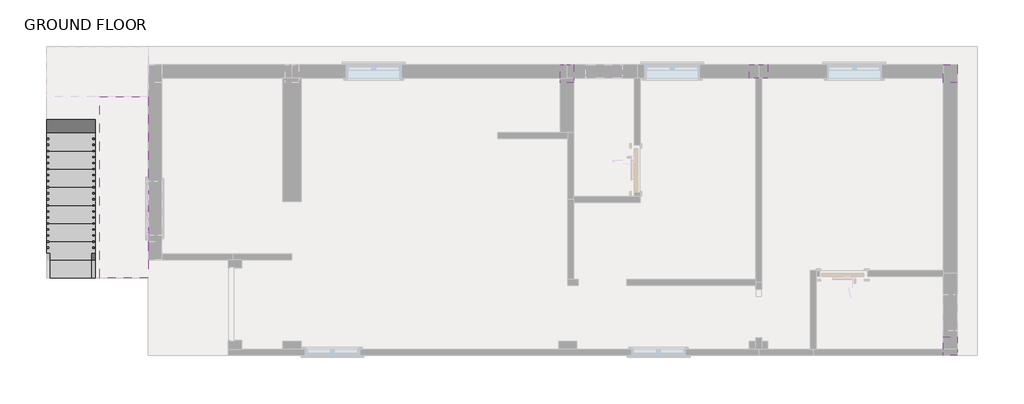
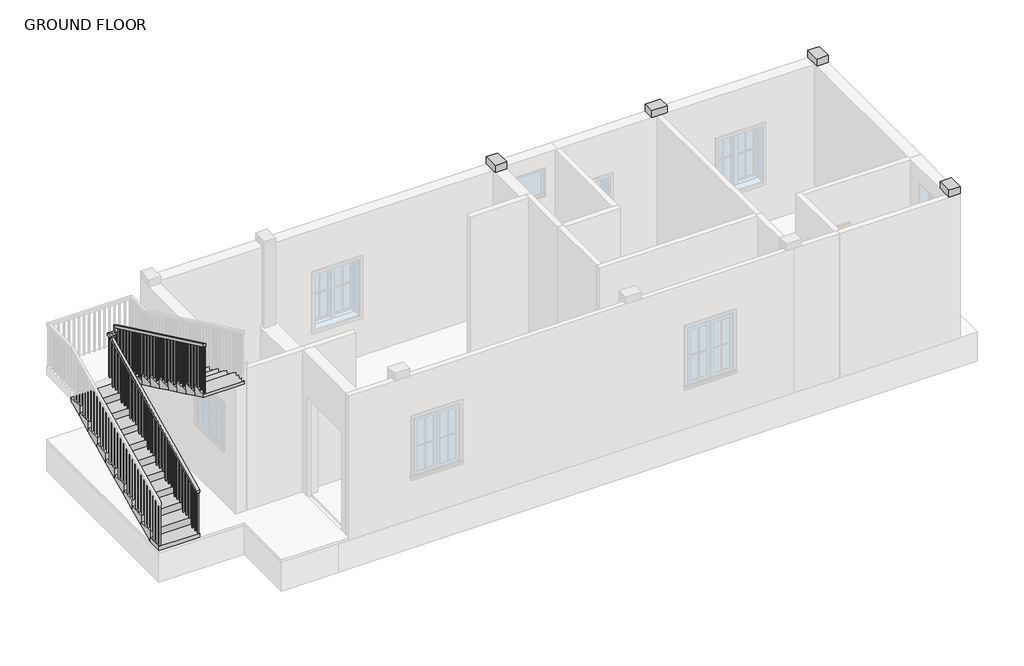
# One storey, part 2 of 3: 4 columns, 2 stair flights, 1 railing.
"""IFC4 building model written with IfcOpenShell, lengths in millimetres."""

from ifc_helpers import new_model, si_unit, frame, origin, place, context, project, spatial, polyline, outline, extrude, faceted_brep, element, save

model = new_model("IFC4")

# Units and contexts
model_context = context("Model", 3, world=origin())
ifc_project = project(units=[si_unit("LENGTHUNIT", "METRE", prefix="MILLI")], contexts=[model_context])

# Site, building, storey
site = spatial("IfcSite", under=ifc_project)
building = spatial("IfcBuilding", under=site)
storey = spatial("IfcBuildingStorey", under=building, Name="GROUND FLOOR", Elevation=0.0)

# Columns
placement = place(None, origin())
element("IfcColumn", 1, ObjectType="Rectangular Column : 9\" X 12\"", at=placement, inside=storey, context=model_context, shape_type="SweptSolid", body=[
    extrude(outline(polyline([(8641.6408773, 5102.5642852), (8870.2408773, 5102.5642852), (8870.2408773, 4797.7642852), (8641.6408773, 4797.7642852), (8641.6408773, 5102.5642852)])), frame((0.0, 0.0, 3048.0), z_axis=(0.0, 0.0, 1.0), x_axis=(1.0, 0.0, 0.0)), (0.0, 0.0, 1.0), 152.4),
])
element("IfcColumn", 2, ObjectType="Rectangular Column : 9\" X 12\"", at=placement, inside=storey, context=model_context, shape_type="SweptSolid", body=[
    extrude(outline(polyline([(3200.4, 5695.2408773), (3200.4, 5390.4408773), (3048.0, 5390.4408773), (3048.0, 5542.8408773), (3048.0, 5695.2408773), (3200.4, 5695.2408773)])), frame((0.0, 4873.9642852, 0.0), z_axis=(0.0, 1.0, 0.0), x_axis=(0.0, 0.0, 1.0)), (0.0, 0.0, 1.0), 228.6),
])
element("IfcColumn", 3, ObjectType="Rectangular Column : 9\" X 12\"", at=placement, inside=storey, context=model_context, shape_type="Brep", body=[
    faceted_brep([(2215.4408773, 5102.5642852, 3200.4), (2444.0408773, 5102.5642852, 3200.4), (2444.0408773, 5102.5642852, 3048.0), (2329.7408773, 5102.5642852, 3048.0), (2215.4408773, 5102.5642852, 3048.0), (2444.0408773, 4797.7642852, 3200.4), (2444.0408773, 4797.7642852, 3048.0), (2444.0408773, 4873.9642852, 3048.0), (2215.4408773, 4797.7642852, 3200.4), (2215.4408773, 4797.7642852, 3048.0), (2215.4408773, 4873.9642852, 3048.0), (2329.7408773, 4873.9642852, 3048.0)], [[[0, 1, 2, 3, 4]], [[1, 5, 6, 7, 2]], [[5, 8, 9, 6]], [[8, 0, 4, 10, 9]], [[1, 0, 8, 5]], [[6, 9, 10, 11, 7]], [[10, 4, 3, 11]], [[3, 2, 7, 11]]]),
])
element("IfcColumn", 4, ObjectType="Rectangular Column : 9\" X 12\"", at=placement, inside=storey, context=model_context, shape_type="SweptSolid", body=[
    extrude(outline(polyline([(225.7642852, 3200.4), (530.5642852, 3200.4), (530.5642852, 3048.0), (327.3642852, 3048.0), (225.7642852, 3048.0), (225.7642852, 3200.4)])), frame((8641.6408773, 0.0, 0.0), z_axis=(1.0, 0.0, 0.0), x_axis=(0.0, 1.0, 0.0)), (0.0, 0.0, 1.0), 228.6),
])

# Railing
element("IfcRailing", 5, ObjectType="Handrail - Rectangular", at=placement, inside=storey, context=model_context, shape_type="SolidModel", body=[
    faceted_brep([(-5633.1591227, 1521.1642852, 1059.8727273), (-5633.1591227, 1521.1642852, 1003.5834559), (-5582.3591227, 1521.1642852, 1003.5834559), (-5582.3591227, 1521.1642852, 1059.8727273), (-5633.1591227, 4492.9642852, 2478.2318182), (-5633.1591227, 4543.7642852, 2446.1880014), (-5582.3591227, 4543.7642852, 2446.1880014), (-5582.3591227, 4492.9642852, 2478.2318182), (-5633.1591227, 4492.9642852, 2514.6), (-5633.1591227, 4543.7642852, 2463.8), (-5582.3591227, 4543.7642852, 2463.8), (-5582.3591227, 4492.9642852, 2514.6), (-5633.1591227, 4619.9642852, 2514.6), (-5633.1591227, 4619.9642852, 2463.8), (-5582.3591227, 4569.1642852, 2463.8), (-5582.3591227, 4569.1642852, 2514.6), (-5506.1591227, 4619.9642852, 2514.6), (-5506.1591227, 4619.9642852, 2463.8), (-5506.1591227, 4569.1642852, 2463.8), (-5506.1591227, 4569.1642852, 2514.6), (-5480.7591227, 4619.9642852, 2514.6), (-5480.7591227, 4569.1642852, 2514.6), (-5480.7591227, 4569.1642852, 2463.8), (-5480.7591227, 4619.9642852, 2463.8)], [[[0, 1, 2, 3]], [[1, 0, 4, 5]], [[2, 1, 5, 6]], [[3, 2, 6, 7]], [[0, 3, 7, 4]], [[5, 4, 8, 9]], [[6, 5, 9, 10]], [[7, 6, 10, 11]], [[4, 7, 11, 8]], [[9, 8, 12, 13]], [[10, 9, 13, 14]], [[11, 10, 14, 15]], [[8, 11, 15, 12]], [[13, 12, 16, 17]], [[14, 13, 17, 18]], [[15, 14, 18, 19]], [[12, 15, 19, 16]], [[20, 21, 22, 23]], [[17, 16, 20, 23]], [[18, 17, 23, 22]], [[19, 18, 22, 21]], [[16, 19, 21, 20]]]),
    faceted_brep([(-5506.1591227, 4619.9642852, 2514.6), (-5455.3591227, 4619.9642852, 2463.8), (-5455.3591227, 4569.1642852, 2463.8), (-5506.1591227, 4569.1642852, 2514.6), (-5506.1591227, 4619.9642852, 2635.8272727), (-5506.1591227, 4569.1642852, 2603.7834559), (-5455.3591227, 4569.1642852, 2603.7834559), (-5455.3591227, 4619.9642852, 2635.8272727)], [[[0, 1, 2, 3]], [[4, 5, 6, 7]], [[1, 0, 4, 7]], [[2, 1, 7, 6]], [[3, 2, 6, 5]], [[0, 3, 5, 4]]]),
    faceted_brep([(-5455.3591227, 4619.9642852, 2635.8272727), (-5455.3591227, 4569.1642852, 2603.7834559), (-5506.1591227, 4569.1642852, 2603.7834559), (-5506.1591227, 4619.9642852, 2635.8272727), (-5455.3591227, 1521.1642852, 4114.8), (-5506.1591227, 1521.1642852, 4114.8), (-5506.1591227, 1521.1642852, 4058.5107287), (-5455.3591227, 1521.1642852, 4058.5107287)], [[[0, 1, 2, 3]], [[4, 5, 6, 7]], [[1, 0, 4, 7]], [[2, 1, 7, 6]], [[3, 2, 6, 5]], [[0, 3, 5, 4]]]),
    extrude(outline(polyline([(1537.0392852, 4050.9340241), (1556.0892852, 4041.8419787), (1556.0892852, 3054.9272727), (1537.0392852, 3054.9272727), (1537.0392852, 4050.9340241)])), frame((-5490.2841227, 0.0, 0.0), z_axis=(1.0, 0.0, 0.0), x_axis=(0.0, 1.0, 0.0)), (0.0, 0.0, 1.0), 19.05),
    extrude(outline(polyline([(1638.6392852, 4002.443115), (1657.6892852, 3993.3510696), (1657.6892852, 3054.9272727), (1638.6392852, 3054.9272727), (1638.6392852, 4002.443115)])), frame((-5490.2841227, 0.0, 0.0), z_axis=(1.0, 0.0, 0.0), x_axis=(0.0, 1.0, 0.0)), (0.0, 0.0, 1.0), 19.05),
    extrude(outline(polyline([(1740.2392852, 3953.9522059), (1759.2892852, 3944.8601605), (1759.2892852, 3054.9272727), (1740.2392852, 3054.9272727), (1740.2392852, 3953.9522059)])), frame((-5490.2841227, 0.0, 0.0), z_axis=(1.0, 0.0, 0.0), x_axis=(0.0, 1.0, 0.0)), (0.0, 0.0, 1.0), 19.05),
    extrude(outline(polyline([(1841.8392852, 3905.4612969), (1860.8892852, 3896.3692514), (1860.8892852, 2909.4545455), (1841.8392852, 2909.4545455), (1841.8392852, 3905.4612969)])), frame((-5490.2841227, 0.0, 0.0), z_axis=(1.0, 0.0, 0.0), x_axis=(0.0, 1.0, 0.0)), (0.0, 0.0, 1.0), 19.05),
    extrude(outline(polyline([(1943.4392852, 3856.9703878), (1962.4892852, 3847.8783423), (1962.4892852, 2909.4545455), (1943.4392852, 2909.4545455), (1943.4392852, 3856.9703878)])), frame((-5490.2841227, 0.0, 0.0), z_axis=(1.0, 0.0, 0.0), x_axis=(0.0, 1.0, 0.0)), (0.0, 0.0, 1.0), 19.05),
    extrude(outline(polyline([(2045.0392852, 3808.4794787), (2064.0892852, 3799.3874332), (2064.0892852, 2909.4545455), (2045.0392852, 2909.4545455), (2045.0392852, 3808.4794787)])), frame((-5490.2841227, 0.0, 0.0), z_axis=(1.0, 0.0, 0.0), x_axis=(0.0, 1.0, 0.0)), (0.0, 0.0, 1.0), 19.05),
    extrude(outline(polyline([(2146.6392852, 3759.9885696), (2165.6892852, 3750.8965241), (2165.6892852, 2763.9818182), (2146.6392852, 2763.9818182), (2146.6392852, 3759.9885696)])), frame((-5490.2841227, 0.0, 0.0), z_axis=(1.0, 0.0, 0.0), x_axis=(0.0, 1.0, 0.0)), (0.0, 0.0, 1.0), 19.05),
    extrude(outline(polyline([(2248.2392852, 3711.4976605), (2267.2892852, 3702.405615), (2267.2892852, 2763.9818182), (2248.2392852, 2763.9818182), (2248.2392852, 3711.4976605)])), frame((-5490.2841227, 0.0, 0.0), z_axis=(1.0, 0.0, 0.0), x_axis=(0.0, 1.0, 0.0)), (0.0, 0.0, 1.0), 19.05),
    extrude(outline(polyline([(2349.8392852, 3663.0067514), (2368.8892852, 3653.9147059), (2368.8892852, 2763.9818182), (2349.8392852, 2763.9818182), (2349.8392852, 3663.0067514)])), frame((-5490.2841227, 0.0, 0.0), z_axis=(1.0, 0.0, 0.0), x_axis=(0.0, 1.0, 0.0)), (0.0, 0.0, 1.0), 19.05),
    extrude(outline(polyline([(2451.4392852, 3614.5158423), (2470.4892852, 3605.4237969), (2470.4892852, 2618.5090909), (2451.4392852, 2618.5090909), (2451.4392852, 3614.5158423)])), frame((-5490.2841227, 0.0, 0.0), z_axis=(1.0, 0.0, 0.0), x_axis=(0.0, 1.0, 0.0)), (0.0, 0.0, 1.0), 19.05),
    extrude(outline(polyline([(2553.0392852, 3566.0249332), (2572.0892852, 3556.9328878), (2572.0892852, 2618.5090909), (2553.0392852, 2618.5090909), (2553.0392852, 3566.0249332)])), frame((-5490.2841227, 0.0, 0.0), z_axis=(1.0, 0.0, 0.0), x_axis=(0.0, 1.0, 0.0)), (0.0, 0.0, 1.0), 19.05),
    extrude(outline(polyline([(2654.6392852, 3517.5340241), (2673.6892852, 3508.4419787), (2673.6892852, 2618.5090909), (2654.6392852, 2618.5090909), (2654.6392852, 3517.5340241)])), frame((-5490.2841227, 0.0, 0.0), z_axis=(1.0, 0.0, 0.0), x_axis=(0.0, 1.0, 0.0)), (0.0, 0.0, 1.0), 19.05),
    extrude(outline(polyline([(2756.2392852, 3469.043115), (2775.2892852, 3459.9510696), (2775.2892852, 2473.0363636), (2756.2392852, 2473.0363636), (2756.2392852, 3469.043115)])), frame((-5490.2841227, 0.0, 0.0), z_axis=(1.0, 0.0, 0.0), x_axis=(0.0, 1.0, 0.0)), (0.0, 0.0, 1.0), 19.05),
    extrude(outline(polyline([(2857.8392852, 3420.5522059), (2876.8892852, 3411.4601605), (2876.8892852, 2473.0363636), (2857.8392852, 2473.0363636), (2857.8392852, 3420.5522059)])), frame((-5490.2841227, 0.0, 0.0), z_axis=(1.0, 0.0, 0.0), x_axis=(0.0, 1.0, 0.0)), (0.0, 0.0, 1.0), 19.05),
    extrude(outline(polyline([(2959.4392852, 3372.0612969), (2978.4892852, 3362.9692514), (2978.4892852, 2473.0363636), (2959.4392852, 2473.0363636), (2959.4392852, 3372.0612969)])), frame((-5490.2841227, 0.0, 0.0), z_axis=(1.0, 0.0, 0.0), x_axis=(0.0, 1.0, 0.0)), (0.0, 0.0, 1.0), 19.05),
    extrude(outline(polyline([(3061.0392852, 3323.5703878), (3080.0892852, 3314.4783423), (3080.0892852, 2327.5636364), (3061.0392852, 2327.5636364), (3061.0392852, 3323.5703878)])), frame((-5490.2841227, 0.0, 0.0), z_axis=(1.0, 0.0, 0.0), x_axis=(0.0, 1.0, 0.0)), (0.0, 0.0, 1.0), 19.05),
    extrude(outline(polyline([(3162.6392852, 3275.0794787), (3181.6892852, 3265.9874332), (3181.6892852, 2327.5636364), (3162.6392852, 2327.5636364), (3162.6392852, 3275.0794787)])), frame((-5490.2841227, 0.0, 0.0), z_axis=(1.0, 0.0, 0.0), x_axis=(0.0, 1.0, 0.0)), (0.0, 0.0, 1.0), 19.05),
    extrude(outline(polyline([(3264.2392852, 3226.5885696), (3283.2892852, 3217.4965241), (3283.2892852, 2327.5636364), (3264.2392852, 2327.5636364), (3264.2392852, 3226.5885696)])), frame((-5490.2841227, 0.0, 0.0), z_axis=(1.0, 0.0, 0.0), x_axis=(0.0, 1.0, 0.0)), (0.0, 0.0, 1.0), 19.05),
    extrude(outline(polyline([(3365.8392852, 3178.0976605), (3384.8892852, 3169.005615), (3384.8892852, 2182.0909091), (3365.8392852, 2182.0909091), (3365.8392852, 3178.0976605)])), frame((-5490.2841227, 0.0, 0.0), z_axis=(1.0, 0.0, 0.0), x_axis=(0.0, 1.0, 0.0)), (0.0, 0.0, 1.0), 19.05),
    extrude(outline(polyline([(3467.4392852, 3129.6067514), (3486.4892852, 3120.5147059), (3486.4892852, 2182.0909091), (3467.4392852, 2182.0909091), (3467.4392852, 3129.6067514)])), frame((-5490.2841227, 0.0, 0.0), z_axis=(1.0, 0.0, 0.0), x_axis=(0.0, 1.0, 0.0)), (0.0, 0.0, 1.0), 19.05),
    extrude(outline(polyline([(3569.0392852, 3081.1158423), (3588.0892852, 3072.0237969), (3588.0892852, 2182.0909091), (3569.0392852, 2182.0909091), (3569.0392852, 3081.1158423)])), frame((-5490.2841227, 0.0, 0.0), z_axis=(1.0, 0.0, 0.0), x_axis=(0.0, 1.0, 0.0)), (0.0, 0.0, 1.0), 19.05),
    extrude(outline(polyline([(3670.6392852, 3032.6249332), (3689.6892852, 3023.5328878), (3689.6892852, 2036.6181818), (3670.6392852, 2036.6181818), (3670.6392852, 3032.6249332)])), frame((-5490.2841227, 0.0, 0.0), z_axis=(1.0, 0.0, 0.0), x_axis=(0.0, 1.0, 0.0)), (0.0, 0.0, 1.0), 19.05),
    extrude(outline(polyline([(3772.2392852, 2984.1340241), (3791.2892852, 2975.0419787), (3791.2892852, 2036.6181818), (3772.2392852, 2036.6181818), (3772.2392852, 2984.1340241)])), frame((-5490.2841227, 0.0, 0.0), z_axis=(1.0, 0.0, 0.0), x_axis=(0.0, 1.0, 0.0)), (0.0, 0.0, 1.0), 19.05),
    extrude(outline(polyline([(3873.8392852, 2935.643115), (3892.8892852, 2926.5510696), (3892.8892852, 2036.6181818), (3873.8392852, 2036.6181818), (3873.8392852, 2935.643115)])), frame((-5490.2841227, 0.0, 0.0), z_axis=(1.0, 0.0, 0.0), x_axis=(0.0, 1.0, 0.0)), (0.0, 0.0, 1.0), 19.05),
    extrude(outline(polyline([(3975.4392852, 2887.1522059), (3994.4892852, 2878.0601605), (3994.4892852, 1891.1454545), (3975.4392852, 1891.1454545), (3975.4392852, 2887.1522059)])), frame((-5490.2841227, 0.0, 0.0), z_axis=(1.0, 0.0, 0.0), x_axis=(0.0, 1.0, 0.0)), (0.0, 0.0, 1.0), 19.05),
    extrude(outline(polyline([(4077.0392852, 2838.6612969), (4096.0892852, 2829.5692514), (4096.0892852, 1891.1454545), (4077.0392852, 1891.1454545), (4077.0392852, 2838.6612969)])), frame((-5490.2841227, 0.0, 0.0), z_axis=(1.0, 0.0, 0.0), x_axis=(0.0, 1.0, 0.0)), (0.0, 0.0, 1.0), 19.05),
    extrude(outline(polyline([(4178.6392852, 2790.1703878), (4197.6892852, 2781.0783423), (4197.6892852, 1891.1454545), (4178.6392852, 1891.1454545), (4178.6392852, 2790.1703878)])), frame((-5490.2841227, 0.0, 0.0), z_axis=(1.0, 0.0, 0.0), x_axis=(0.0, 1.0, 0.0)), (0.0, 0.0, 1.0), 19.05),
    extrude(outline(polyline([(4280.2392852, 2741.6794787), (4299.2892852, 2732.5874332), (4299.2892852, 1745.6727273), (4280.2392852, 1745.6727273), (4280.2392852, 2741.6794787)])), frame((-5490.2841227, 0.0, 0.0), z_axis=(1.0, 0.0, 0.0), x_axis=(0.0, 1.0, 0.0)), (0.0, 0.0, 1.0), 19.05),
    extrude(outline(polyline([(4381.8392852, 2693.1885696), (4400.8892852, 2684.0965241), (4400.8892852, 1745.6727273), (4381.8392852, 1745.6727273), (4381.8392852, 2693.1885696)])), frame((-5490.2841227, 0.0, 0.0), z_axis=(1.0, 0.0, 0.0), x_axis=(0.0, 1.0, 0.0)), (0.0, 0.0, 1.0), 19.05),
    extrude(outline(polyline([(4483.4392852, 2644.6976605), (4502.4892852, 2635.605615), (4502.4892852, 1745.6727273), (4483.4392852, 1745.6727273), (4483.4392852, 2644.6976605)])), frame((-5490.2841227, 0.0, 0.0), z_axis=(1.0, 0.0, 0.0), x_axis=(0.0, 1.0, 0.0)), (0.0, 0.0, 1.0), 19.05),
    extrude(outline(polyline([(-5515.6841227, 4585.0392852), (-5515.6841227, 4604.0892852), (-5496.6341227, 4604.0892852), (-5496.6341227, 4585.0392852), (-5515.6841227, 4585.0392852)])), frame((0.0, 0.0, 1600.2), z_axis=(0.0, 0.0, 1.0), x_axis=(1.0, 0.0, 0.0)), (0.0, 0.0, 1.0), 863.6),
    extrude(outline(polyline([(-5598.2341227, 4559.6392852), (-5617.2841227, 4559.6392852), (-5617.2841227, 4578.6892852), (-5598.2341227, 4578.6892852), (-5598.2341227, 4559.6392852)])), frame((0.0, 0.0, 1600.2), z_axis=(0.0, 0.0, 1.0), x_axis=(1.0, 0.0, 0.0)), (0.0, 0.0, 1.0), 863.6),
    extrude(outline(polyline([(4458.0392852, 2405.2737969), (4477.0892852, 2414.3658423), (4477.0892852, 1454.7272727), (4458.0392852, 1454.7272727), (4458.0392852, 2405.2737969)])), frame((-5617.2841227, 0.0, 0.0), z_axis=(1.0, 0.0, 0.0), x_axis=(0.0, 1.0, 0.0)), (0.0, 0.0, 1.0), 19.05),
    extrude(outline(polyline([(4356.4392852, 2356.7828878), (4375.4892852, 2365.8749332), (4375.4892852, 1454.7272727), (4356.4392852, 1454.7272727), (4356.4392852, 2356.7828878)])), frame((-5617.2841227, 0.0, 0.0), z_axis=(1.0, 0.0, 0.0), x_axis=(0.0, 1.0, 0.0)), (0.0, 0.0, 1.0), 19.05),
    extrude(outline(polyline([(4254.8392852, 2308.2919787), (4273.8892852, 2317.3840241), (4273.8892852, 1454.7272727), (4254.8392852, 1454.7272727), (4254.8392852, 2308.2919787)])), frame((-5617.2841227, 0.0, 0.0), z_axis=(1.0, 0.0, 0.0), x_axis=(0.0, 1.0, 0.0)), (0.0, 0.0, 1.0), 19.05),
    extrude(outline(polyline([(4153.2392852, 2259.8010696), (4172.2892852, 2268.893115), (4172.2892852, 1309.2545455), (4153.2392852, 1309.2545455), (4153.2392852, 2259.8010696)])), frame((-5617.2841227, 0.0, 0.0), z_axis=(1.0, 0.0, 0.0), x_axis=(0.0, 1.0, 0.0)), (0.0, 0.0, 1.0), 19.05),
    extrude(outline(polyline([(4051.6392852, 2211.3101605), (4070.6892852, 2220.4022059), (4070.6892852, 1309.2545455), (4051.6392852, 1309.2545455), (4051.6392852, 2211.3101605)])), frame((-5617.2841227, 0.0, 0.0), z_axis=(1.0, 0.0, 0.0), x_axis=(0.0, 1.0, 0.0)), (0.0, 0.0, 1.0), 19.05),
    extrude(outline(polyline([(3950.0392852, 2162.8192514), (3969.0892852, 2171.9112969), (3969.0892852, 1309.2545455), (3950.0392852, 1309.2545455), (3950.0392852, 2162.8192514)])), frame((-5617.2841227, 0.0, 0.0), z_axis=(1.0, 0.0, 0.0), x_axis=(0.0, 1.0, 0.0)), (0.0, 0.0, 1.0), 19.05),
    extrude(outline(polyline([(3848.4392852, 2114.3283423), (3867.4892852, 2123.4203878), (3867.4892852, 1163.7818182), (3848.4392852, 1163.7818182), (3848.4392852, 2114.3283423)])), frame((-5617.2841227, 0.0, 0.0), z_axis=(1.0, 0.0, 0.0), x_axis=(0.0, 1.0, 0.0)), (0.0, 0.0, 1.0), 19.05),
    extrude(outline(polyline([(3746.8392852, 2065.8374332), (3765.8892852, 2074.9294787), (3765.8892852, 1163.7818182), (3746.8392852, 1163.7818182), (3746.8392852, 2065.8374332)])), frame((-5617.2841227, 0.0, 0.0), z_axis=(1.0, 0.0, 0.0), x_axis=(0.0, 1.0, 0.0)), (0.0, 0.0, 1.0), 19.05),
    extrude(outline(polyline([(3645.2392852, 2017.3465241), (3664.2892852, 2026.4385696), (3664.2892852, 1163.7818182), (3645.2392852, 1163.7818182), (3645.2392852, 2017.3465241)])), frame((-5617.2841227, 0.0, 0.0), z_axis=(1.0, 0.0, 0.0), x_axis=(0.0, 1.0, 0.0)), (0.0, 0.0, 1.0), 19.05),
    extrude(outline(polyline([(3543.6392852, 1968.855615), (3562.6892852, 1977.9476605), (3562.6892852, 1018.3090909), (3543.6392852, 1018.3090909), (3543.6392852, 1968.855615)])), frame((-5617.2841227, 0.0, 0.0), z_axis=(1.0, 0.0, 0.0), x_axis=(0.0, 1.0, 0.0)), (0.0, 0.0, 1.0), 19.05),
    extrude(outline(polyline([(3442.0392852, 1920.3647059), (3461.0892852, 1929.4567514), (3461.0892852, 1018.3090909), (3442.0392852, 1018.3090909), (3442.0392852, 1920.3647059)])), frame((-5617.2841227, 0.0, 0.0), z_axis=(1.0, 0.0, 0.0), x_axis=(0.0, 1.0, 0.0)), (0.0, 0.0, 1.0), 19.05),
    extrude(outline(polyline([(3340.4392852, 1871.8737969), (3359.4892852, 1880.9658423), (3359.4892852, 1018.3090909), (3340.4392852, 1018.3090909), (3340.4392852, 1871.8737969)])), frame((-5617.2841227, 0.0, 0.0), z_axis=(1.0, 0.0, 0.0), x_axis=(0.0, 1.0, 0.0)), (0.0, 0.0, 1.0), 19.05),
    extrude(outline(polyline([(3238.8392852, 1823.3828878), (3257.8892852, 1832.4749332), (3257.8892852, 872.8363636), (3238.8392852, 872.8363636), (3238.8392852, 1823.3828878)])), frame((-5617.2841227, 0.0, 0.0), z_axis=(1.0, 0.0, 0.0), x_axis=(0.0, 1.0, 0.0)), (0.0, 0.0, 1.0), 19.05),
    extrude(outline(polyline([(3137.2392852, 1774.8919787), (3156.2892852, 1783.9840241), (3156.2892852, 872.8363636), (3137.2392852, 872.8363636), (3137.2392852, 1774.8919787)])), frame((-5617.2841227, 0.0, 0.0), z_axis=(1.0, 0.0, 0.0), x_axis=(0.0, 1.0, 0.0)), (0.0, 0.0, 1.0), 19.05),
    extrude(outline(polyline([(3035.6392852, 1726.4010696), (3054.6892852, 1735.493115), (3054.6892852, 872.8363636), (3035.6392852, 872.8363636), (3035.6392852, 1726.4010696)])), frame((-5617.2841227, 0.0, 0.0), z_axis=(1.0, 0.0, 0.0), x_axis=(0.0, 1.0, 0.0)), (0.0, 0.0, 1.0), 19.05),
    extrude(outline(polyline([(2934.0392852, 1677.9101605), (2953.0892852, 1687.0022059), (2953.0892852, 727.3636364), (2934.0392852, 727.3636364), (2934.0392852, 1677.9101605)])), frame((-5617.2841227, 0.0, 0.0), z_axis=(1.0, 0.0, 0.0), x_axis=(0.0, 1.0, 0.0)), (0.0, 0.0, 1.0), 19.05),
    extrude(outline(polyline([(2832.4392852, 1629.4192514), (2851.4892852, 1638.5112969), (2851.4892852, 727.3636364), (2832.4392852, 727.3636364), (2832.4392852, 1629.4192514)])), frame((-5617.2841227, 0.0, 0.0), z_axis=(1.0, 0.0, 0.0), x_axis=(0.0, 1.0, 0.0)), (0.0, 0.0, 1.0), 19.05),
    extrude(outline(polyline([(2730.8392852, 1580.9283423), (2749.8892852, 1590.0203878), (2749.8892852, 727.3636364), (2730.8392852, 727.3636364), (2730.8392852, 1580.9283423)])), frame((-5617.2841227, 0.0, 0.0), z_axis=(1.0, 0.0, 0.0), x_axis=(0.0, 1.0, 0.0)), (0.0, 0.0, 1.0), 19.05),
    extrude(outline(polyline([(2629.2392852, 1532.4374332), (2648.2892852, 1541.5294787), (2648.2892852, 581.8909091), (2629.2392852, 581.8909091), (2629.2392852, 1532.4374332)])), frame((-5617.2841227, 0.0, 0.0), z_axis=(1.0, 0.0, 0.0), x_axis=(0.0, 1.0, 0.0)), (0.0, 0.0, 1.0), 19.05),
    extrude(outline(polyline([(2527.6392852, 1483.9465241), (2546.6892852, 1493.0385696), (2546.6892852, 581.8909091), (2527.6392852, 581.8909091), (2527.6392852, 1483.9465241)])), frame((-5617.2841227, 0.0, 0.0), z_axis=(1.0, 0.0, 0.0), x_axis=(0.0, 1.0, 0.0)), (0.0, 0.0, 1.0), 19.05),
    extrude(outline(polyline([(2426.0392852, 1435.455615), (2445.0892852, 1444.5476605), (2445.0892852, 581.8909091), (2426.0392852, 581.8909091), (2426.0392852, 1435.455615)])), frame((-5617.2841227, 0.0, 0.0), z_axis=(1.0, 0.0, 0.0), x_axis=(0.0, 1.0, 0.0)), (0.0, 0.0, 1.0), 19.05),
    extrude(outline(polyline([(2324.4392852, 1386.9647059), (2343.4892852, 1396.0567514), (2343.4892852, 436.4181818), (2324.4392852, 436.4181818), (2324.4392852, 1386.9647059)])), frame((-5617.2841227, 0.0, 0.0), z_axis=(1.0, 0.0, 0.0), x_axis=(0.0, 1.0, 0.0)), (0.0, 0.0, 1.0), 19.05),
    extrude(outline(polyline([(2222.8392852, 1338.4737969), (2241.8892852, 1347.5658423), (2241.8892852, 436.4181818), (2222.8392852, 436.4181818), (2222.8392852, 1338.4737969)])), frame((-5617.2841227, 0.0, 0.0), z_axis=(1.0, 0.0, 0.0), x_axis=(0.0, 1.0, 0.0)), (0.0, 0.0, 1.0), 19.05),
    extrude(outline(polyline([(2121.2392852, 1289.9828878), (2140.2892852, 1299.0749332), (2140.2892852, 436.4181818), (2121.2392852, 436.4181818), (2121.2392852, 1289.9828878)])), frame((-5617.2841227, 0.0, 0.0), z_axis=(1.0, 0.0, 0.0), x_axis=(0.0, 1.0, 0.0)), (0.0, 0.0, 1.0), 19.05),
    extrude(outline(polyline([(2019.6392852, 1241.4919787), (2038.6892852, 1250.5840241), (2038.6892852, 290.9454545), (2019.6392852, 290.9454545), (2019.6392852, 1241.4919787)])), frame((-5617.2841227, 0.0, 0.0), z_axis=(1.0, 0.0, 0.0), x_axis=(0.0, 1.0, 0.0)), (0.0, 0.0, 1.0), 19.05),
    extrude(outline(polyline([(1918.0392852, 1193.0010696), (1937.0892852, 1202.093115), (1937.0892852, 290.9454545), (1918.0392852, 290.9454545), (1918.0392852, 1193.0010696)])), frame((-5617.2841227, 0.0, 0.0), z_axis=(1.0, 0.0, 0.0), x_axis=(0.0, 1.0, 0.0)), (0.0, 0.0, 1.0), 19.05),
    extrude(outline(polyline([(1816.4392852, 1144.5101605), (1835.4892852, 1153.6022059), (1835.4892852, 290.9454545), (1816.4392852, 290.9454545), (1816.4392852, 1144.5101605)])), frame((-5617.2841227, 0.0, 0.0), z_axis=(1.0, 0.0, 0.0), x_axis=(0.0, 1.0, 0.0)), (0.0, 0.0, 1.0), 19.05),
    extrude(outline(polyline([(1714.8392852, 1096.0192514), (1733.8892852, 1105.1112969), (1733.8892852, 145.4727273), (1714.8392852, 145.4727273), (1714.8392852, 1096.0192514)])), frame((-5617.2841227, 0.0, 0.0), z_axis=(1.0, 0.0, 0.0), x_axis=(0.0, 1.0, 0.0)), (0.0, 0.0, 1.0), 19.05),
    extrude(outline(polyline([(1613.2392852, 1047.5283423), (1632.2892852, 1056.6203878), (1632.2892852, 145.4727273), (1613.2392852, 145.4727273), (1613.2392852, 1047.5283423)])), frame((-5617.2841227, 0.0, 0.0), z_axis=(1.0, 0.0, 0.0), x_axis=(0.0, 1.0, 0.0)), (0.0, 0.0, 1.0), 19.05),
    extrude(outline(polyline([(-5490.2841227, 4585.0392852), (-5490.2841227, 4604.0892852), (-5471.2341227, 4604.0892852), (-5471.2341227, 4585.0392852), (-5490.2841227, 4585.0392852)])), frame((0.0, 0.0, 1600.2), z_axis=(0.0, 0.0, 1.0), x_axis=(1.0, 0.0, 0.0)), (0.0, 0.0, 1.0), 863.6),
    extrude(outline(polyline([(-5598.2341227, 4585.0392852), (-5617.2841227, 4585.0392852), (-5617.2841227, 4604.0892852), (-5598.2341227, 4604.0892852), (-5598.2341227, 4585.0392852)])), frame((0.0, 0.0, 1600.2), z_axis=(0.0, 0.0, 1.0), x_axis=(1.0, 0.0, 0.0)), (0.0, 0.0, 1.0), 863.6),
    extrude(outline(polyline([(1521.1642852, 4058.5107287), (1540.2142852, 4049.4186832), (1540.2142852, 3054.9272727), (1521.1642852, 3054.9272727), (1521.1642852, 4058.5107287)])), frame((-5490.2841227, 0.0, 0.0), z_axis=(1.0, 0.0, 0.0), x_axis=(0.0, 1.0, 0.0)), (0.0, 0.0, 1.0), 19.05),
    extrude(outline(polyline([(1521.1642852, 1003.5834559), (1540.2142852, 1012.6755014), (1540.2142852, 145.4727273), (1521.1642852, 145.4727273), (1521.1642852, 1003.5834559)])), frame((-5617.2841227, 0.0, 0.0), z_axis=(1.0, 0.0, 0.0), x_axis=(0.0, 1.0, 0.0)), (0.0, 0.0, 1.0), 19.05),
])

# Stair flights
element("IfcStairFlight", 6, ObjectType="3/4\" Nosing", at=placement, inside=storey, context=model_context, shape_type="Brep", body=[
    faceted_brep([(-6395.1591227, 1825.9642852, 145.4727273), (-6395.1591227, 1521.1642852, 145.4727273), (-5582.3591227, 1521.1642852, 145.4727273), (-5582.3591227, 1825.9642852, 145.4727273), (-6395.1591227, 1825.9642852, 75.1111381), (-6395.1591227, 1668.5885672, 0.0), (-6395.1591227, 1521.1642852, 0.0), (-5582.3591227, 1521.1642852, 0.0), (-5582.3591227, 1668.5885672, 0.0), (-5582.3591227, 1825.9642852, 75.1111381), (-6395.1591227, 2130.7642852, 290.9454545), (-6395.1591227, 1825.9642852, 290.9454545), (-5582.3591227, 1825.9642852, 290.9454545), (-5582.3591227, 2130.7642852, 290.9454545), (-6395.1591227, 2130.7642852, 220.5838654), (-5582.3591227, 2130.7642852, 220.5838654), (-6395.1591227, 2435.5642852, 436.4181818), (-6395.1591227, 2130.7642852, 436.4181818), (-5582.3591227, 2130.7642852, 436.4181818), (-5582.3591227, 2435.5642852, 436.4181818), (-6395.1591227, 2435.5642852, 366.0565927), (-5582.3591227, 2435.5642852, 366.0565927), (-6395.1591227, 2740.3642852, 581.8909091), (-6395.1591227, 2435.5642852, 581.8909091), (-5582.3591227, 2435.5642852, 581.8909091), (-5582.3591227, 2740.3642852, 581.8909091), (-6395.1591227, 2740.3642852, 511.5293199), (-5582.3591227, 2740.3642852, 511.5293199), (-6395.1591227, 3045.1642852, 727.3636364), (-6395.1591227, 2740.3642852, 727.3636364), (-5582.3591227, 2740.3642852, 727.3636364), (-5582.3591227, 3045.1642852, 727.3636364), (-6395.1591227, 3045.1642852, 657.0020472), (-5582.3591227, 3045.1642852, 657.0020472), (-6395.1591227, 3349.9642852, 872.8363636), (-6395.1591227, 3045.1642852, 872.8363636), (-5582.3591227, 3045.1642852, 872.8363636), (-5582.3591227, 3349.9642852, 872.8363636), (-6395.1591227, 3349.9642852, 802.4747745), (-5582.3591227, 3349.9642852, 802.4747745), (-6395.1591227, 3654.7642852, 1018.3090909), (-6395.1591227, 3349.9642852, 1018.3090909), (-5582.3591227, 3349.9642852, 1018.3090909), (-5582.3591227, 3654.7642852, 1018.3090909), (-6395.1591227, 3654.7642852, 947.9475018), (-5582.3591227, 3654.7642852, 947.9475018), (-6395.1591227, 3959.5642852, 1163.7818182), (-6395.1591227, 3654.7642852, 1163.7818182), (-5582.3591227, 3654.7642852, 1163.7818182), (-5582.3591227, 3959.5642852, 1163.7818182), (-6395.1591227, 3959.5642852, 1093.420229), (-5582.3591227, 3959.5642852, 1093.420229), (-6395.1591227, 4264.3642852, 1238.8929563), (-6395.1591227, 4569.1642852, 1384.3656836), (-5582.3591227, 4569.1642852, 1384.3656836), (-5582.3591227, 4264.3642852, 1238.8929563), (-6395.1591227, 4264.3642852, 1309.2545455), (-6395.1591227, 3959.5642852, 1309.2545455), (-5582.3591227, 3959.5642852, 1309.2545455), (-5582.3591227, 4264.3642852, 1309.2545455), (-6395.1591227, 4569.1642852, 1454.7272727), (-6395.1591227, 4264.3642852, 1454.7272727), (-5582.3591227, 4264.3642852, 1454.7272727), (-5582.3591227, 4569.1642852, 1454.7272727), (-5582.3591227, 4569.1642852, 1422.4)], [[[0, 1, 2, 3]], [[1, 0, 4, 5, 6]], [[2, 1, 6, 7]], [[3, 2, 7, 8, 9]], [[10, 11, 12, 13]], [[11, 10, 14, 4, 0]], [[0, 3, 12, 11]], [[13, 12, 3, 9, 15]], [[16, 17, 18, 19]], [[17, 16, 20, 14, 10]], [[10, 13, 18, 17]], [[19, 18, 13, 15, 21]], [[22, 23, 24, 25]], [[23, 22, 26, 20, 16]], [[16, 19, 24, 23]], [[25, 24, 19, 21, 27]], [[28, 29, 30, 31]], [[29, 28, 32, 26, 22]], [[22, 25, 30, 29]], [[31, 30, 25, 27, 33]], [[34, 35, 36, 37]], [[35, 34, 38, 32, 28]], [[28, 31, 36, 35]], [[37, 36, 31, 33, 39]], [[40, 41, 42, 43]], [[41, 40, 44, 38, 34]], [[34, 37, 42, 41]], [[43, 42, 37, 39, 45]], [[46, 47, 48, 49]], [[47, 46, 50, 44, 40]], [[40, 43, 48, 47]], [[49, 48, 43, 45, 51]], [[7, 6, 5, 8]], [[8, 5, 4, 14, 20, 26, 32, 38, 44, 50, 52, 53, 54, 55, 51, 45, 39, 33, 27, 21, 15, 9]], [[56, 57, 58, 59]], [[57, 56, 52, 50, 46]], [[46, 49, 58, 57]], [[59, 58, 49, 51, 55]], [[60, 61, 62, 63]], [[61, 60, 53, 52, 56]], [[56, 59, 62, 61]], [[63, 62, 59, 55, 54, 64]], [[60, 63, 64, 54, 53]]]),
])
element("IfcStairFlight", 7, ObjectType="3/4\" Nosing", at=placement, inside=storey, context=model_context, shape_type="Brep", body=[
    faceted_brep([(-4693.3591227, 4264.3642852, 1745.6727273), (-4693.3591227, 4569.1642852, 1745.6727273), (-5506.1591227, 4569.1642852, 1745.6727273), (-5506.1591227, 4264.3642852, 1745.6727273), (-4693.3591227, 4264.3642852, 1675.3111381), (-4693.3591227, 4569.1642852, 1529.8384108), (-4693.3591227, 4569.1642852, 1600.2), (-5506.1591227, 4569.1642852, 1529.8384108), (-5506.1591227, 4264.3642852, 1675.3111381), (-4693.3591227, 3959.5642852, 1891.1454545), (-4693.3591227, 4264.3642852, 1891.1454545), (-5506.1591227, 4264.3642852, 1891.1454545), (-5506.1591227, 3959.5642852, 1891.1454545), (-4693.3591227, 3959.5642852, 1820.7838654), (-5506.1591227, 3959.5642852, 1820.7838654), (-4693.3591227, 3654.7642852, 2036.6181818), (-4693.3591227, 3959.5642852, 2036.6181818), (-5506.1591227, 3959.5642852, 2036.6181818), (-5506.1591227, 3654.7642852, 2036.6181818), (-4693.3591227, 3654.7642852, 1966.2565927), (-5506.1591227, 3654.7642852, 1966.2565927), (-4693.3591227, 3349.9642852, 2182.0909091), (-4693.3591227, 3654.7642852, 2182.0909091), (-5506.1591227, 3654.7642852, 2182.0909091), (-5506.1591227, 3349.9642852, 2182.0909091), (-4693.3591227, 3349.9642852, 2111.7293199), (-5506.1591227, 3349.9642852, 2111.7293199), (-4693.3591227, 3045.1642852, 2327.5636364), (-4693.3591227, 3349.9642852, 2327.5636364), (-5506.1591227, 3349.9642852, 2327.5636364), (-5506.1591227, 3045.1642852, 2327.5636364), (-4693.3591227, 3045.1642852, 2257.2020472), (-5506.1591227, 3045.1642852, 2257.2020472), (-4693.3591227, 2740.3642852, 2473.0363636), (-4693.3591227, 3045.1642852, 2473.0363636), (-5506.1591227, 3045.1642852, 2473.0363636), (-5506.1591227, 2740.3642852, 2473.0363636), (-4693.3591227, 2740.3642852, 2402.6747745), (-5506.1591227, 2740.3642852, 2402.6747745), (-4693.3591227, 2435.5642852, 2618.5090909), (-4693.3591227, 2740.3642852, 2618.5090909), (-5506.1591227, 2740.3642852, 2618.5090909), (-5506.1591227, 2435.5642852, 2618.5090909), (-4693.3591227, 2435.5642852, 2548.1475018), (-5506.1591227, 2435.5642852, 2548.1475018), (-4693.3591227, 2130.7642852, 2763.9818182), (-4693.3591227, 2435.5642852, 2763.9818182), (-5506.1591227, 2435.5642852, 2763.9818182), (-5506.1591227, 2130.7642852, 2763.9818182), (-4693.3591227, 2130.7642852, 2693.620229), (-5506.1591227, 2130.7642852, 2693.620229), (-4693.3591227, 1825.9642852, 2839.0929563), (-4693.3591227, 1521.1642852, 2984.5656836), (-5506.1591227, 1521.1642852, 2984.5656836), (-5506.1591227, 1825.9642852, 2839.0929563), (-4693.3591227, 1825.9642852, 2909.4545455), (-4693.3591227, 2130.7642852, 2909.4545455), (-5506.1591227, 2130.7642852, 2909.4545455), (-5506.1591227, 1825.9642852, 2909.4545455), (-4693.3591227, 1521.1642852, 3054.9272727), (-4693.3591227, 1825.9642852, 3054.9272727), (-5506.1591227, 1825.9642852, 3054.9272727), (-5506.1591227, 1521.1642852, 3054.9272727)], [[[0, 1, 2, 3]], [[1, 0, 4, 5, 6]], [[2, 1, 6, 5, 7]], [[3, 2, 7, 8]], [[9, 10, 11, 12]], [[10, 9, 13, 4, 0]], [[11, 10, 0, 3]], [[12, 11, 3, 8, 14]], [[15, 16, 17, 18]], [[16, 15, 19, 13, 9]], [[17, 16, 9, 12]], [[18, 17, 12, 14, 20]], [[21, 22, 23, 24]], [[22, 21, 25, 19, 15]], [[23, 22, 15, 18]], [[24, 23, 18, 20, 26]], [[27, 28, 29, 30]], [[28, 27, 31, 25, 21]], [[29, 28, 21, 24]], [[30, 29, 24, 26, 32]], [[33, 34, 35, 36]], [[34, 33, 37, 31, 27]], [[35, 34, 27, 30]], [[36, 35, 30, 32, 38]], [[39, 40, 41, 42]], [[40, 39, 43, 37, 33]], [[41, 40, 33, 36]], [[42, 41, 36, 38, 44]], [[45, 46, 47, 48]], [[46, 45, 49, 43, 39]], [[47, 46, 39, 42]], [[48, 47, 42, 44, 50]], [[5, 4, 13, 19, 25, 31, 37, 43, 49, 51, 52, 53, 54, 50, 44, 38, 32, 26, 20, 14, 8, 7]], [[55, 56, 57, 58]], [[56, 55, 51, 49, 45]], [[57, 56, 45, 48]], [[58, 57, 48, 50, 54]], [[59, 60, 61, 62]], [[60, 59, 52, 51, 55]], [[61, 60, 55, 58]], [[62, 61, 58, 54, 53]], [[59, 62, 53, 52]]]),
])

save(model, "model.ifc")

# Revit data of these elements
# Type "Rectangular Column : 9\" X 12\""
#   Assembly Code = "B1010200"
#   Depth = 0' - 9"
#   Offset Base = 0' - 0"
#   Offset Top = 0' - 0"
#   Width = 1' - 0"
#   Material = none
# Type "Handrail - Rectangular"
#   Assembly Code = "C2010400"
#   built-in parameter 1008612 = 0.0416667 (stored number, unit not read)
#   built-in parameter 1008611 = 0.0416667 (stored number, unit not read)
#   built-in parameter 1008609 = 0.333333 (stored number, unit not read)
#   built-in parameter 1008604 = 0.166667 (stored number, unit not read)
#   built-in parameter 1008603 = 0.166667 (stored number, unit not read)
#   Railing Height = 3' - 0"
#   built-in parameter 1008630 = 2
#   built-in parameter 1008610 = 2
#   built-in parameter 1008618 = Baluster - Square : 3/4"
# Elements 1, 2, 3, 4 (IfcColumn, "Rectangular Column : 9\" X 12\"")
#   Phase Created = New Construction
#   Materials on its faces: "Brick, Common"
# Element 5 (IfcRailing, "Handrail - Rectangular")
#   Phase Created = New Construction
# Elements 6, 7 (IfcStairFlight, "3/4\" Nosing")
#   Phase Created = New Construction
#   Materials on its faces: "Concrete, Cast-in-Place gray"
# Materials
#   "Brick, Common": class "Masonry", colour RGB 170 98 104, transparency 0, Description = "Common brick", Cost = 0
#   "Concrete, Cast-in-Place gray": class "Concrete", colour RGB 192 192 192, transparency 0, Description = "Cast-in-place concrete", Cost = 0
